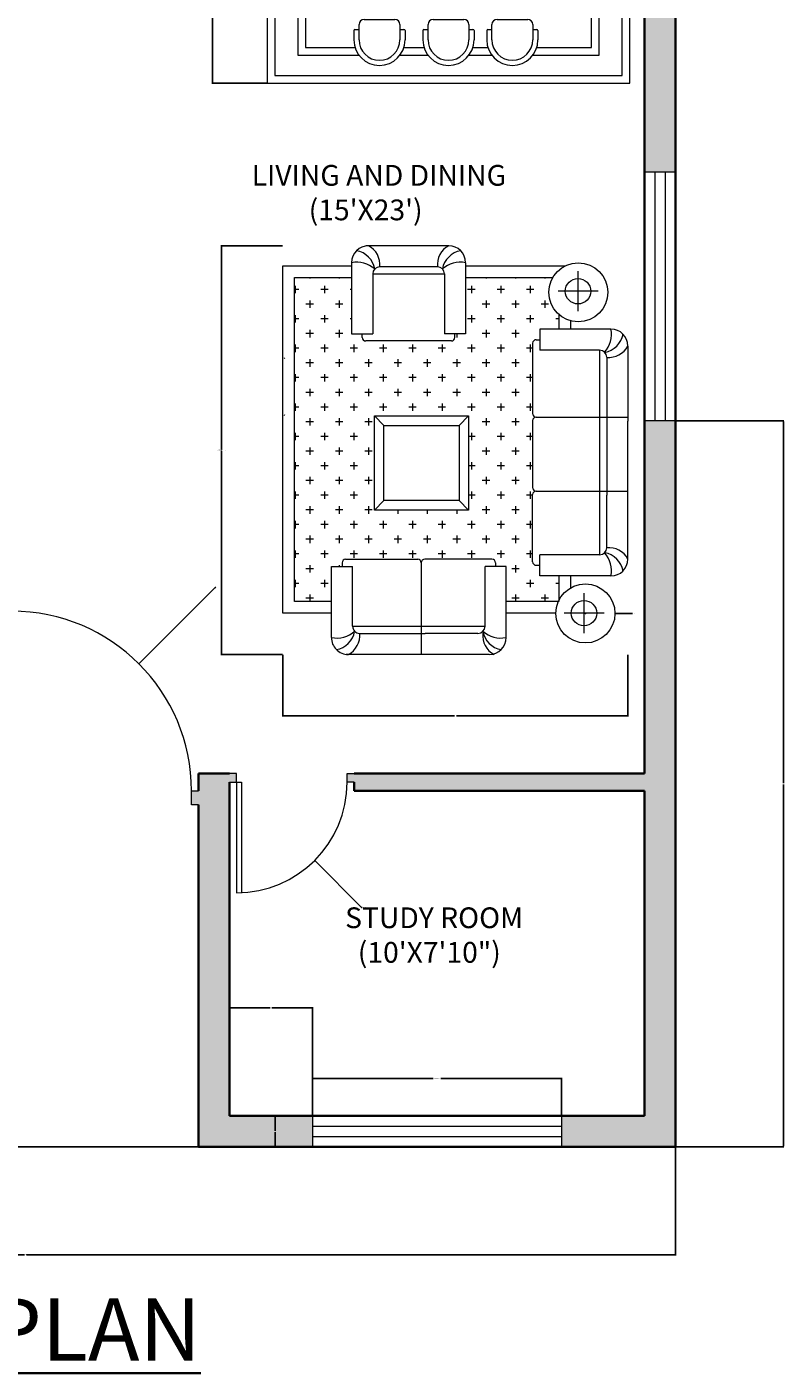
# Model space of a CAD drawing. Units: inches. Extents: x 2948 to 4025, y 2171 to 2966.
# Tile 2 of 6: x 3168 to 3387, y 2171 to 2560. Entities that reach past the tile are written whole.
import ezdxf

# ---------------------------------------------------------------- set-up
doc = ezdxf.new("R2010")
doc.units = ezdxf.units.IN
for name, color, linetype, lineweight in [('A-ANNO-DIMS', 2, 'Continuous', 18), ('A-ANNO-TEXT', 7, 'Continuous', 35), ('A-AREA-IDEN', 7, 'Continuous', 18), ('A-DOOR', 3, 'Continuous', 18), ('A-FURN', 8, 'Continuous', 18), ('A-GLAZ', 4, 'Continuous', 18), ('A-WALL', 7, 'Continuous', 35), ('A-WALL-PATT', 252, 'Continuous', 13)]:
    doc.layers.add(name, color=color, linetype=linetype, lineweight=lineweight)
doc.styles.get("Standard").update_dxf_attribs({"font": 'arial.ttf'})
doc.dimstyles.get("Standard").update_dxf_attribs({"dimtxt": 0.18, "dimasz": 0.18, "dimexe": 0.18, "dimexo": 0.0625, "dimgap": 0.09, "dimtad": 0, "dimtih": 1, "dimtoh": 1, "dimdec": 4, "dimzin": 0, "dimdsep": 46, "dimtxsty": 'Standard', "dimcen": 0.09, "dimadec": 0, "dimazin": 0, "dimtfac": 1, "dimtdec": 4, "dimtofl": 0, "dimtmove": 0, "dimatfit": 3, "dimfxl": 1, "dimtolj": 1, "dimtzin": 0, "dimarcsym": 0})

# ---------------------------------------------------------------- blocks, each defined once
blk = doc.blocks.new('A$C27801A2F')
for p, q in [((3.55, 2.425), (0, 2.425)), ((0, 2.425), (0, 0)), ((3.55, 0), (3.55, 2.425)), ((3.475, 2.35), (0.075, 2.35)), ((0.075, 2.35), (0.075, 0.075)), ((3.475, 0.075), (3.475, 2.35)), ((0.9, 2.125), (0.3, 2.125)), ((0.3, 2.125), (0.3, 1.325)), ((1.575, 2.125), (1.3, 2.125)), ((2.2, 2.125), (1.975, 2.125)), ((3.25, 2.125), (2.6, 2.125)), ((3.25, 1.325), (3.25, 2.125)), ((0.375, 2.05), (0.375, 1.392)), ((0.862, 2.05), (0.375, 2.05)), ((1.537, 2.05), (1.338, 2.05)), ((2.162, 2.05), (2.013, 2.05)), ((3.175, 2.05), (2.638, 2.05)), ((3.175, 1.392), (3.175, 2.05)), ((0.85, 1.885), (0.85, 1.975)), ((0.86, 1.875), (0.9, 1.875)), ((0.9, 1.975), (0.9, 1.825)), ((1.3, 1.825), (1.3, 1.975)), ((1.3, 1.875), (1.34, 1.875)), ((1.35, 1.885), (1.35, 1.975)), ((1.525, 1.885), (1.525, 1.975)), ((1.535, 1.875), (1.575, 1.875)), ((1.575, 1.975), (1.575, 1.825)), ((1.975, 1.825), (1.975, 1.975)), ((1.975, 1.875), (2.015, 1.875)), ((2.025, 1.885), (2.025, 1.975)), ((2.15, 1.885), (2.15, 1.975)), ((2.16, 1.875), (2.2, 1.875)), ((2.2, 1.975), (2.2, 1.825)), ((2.6, 1.825), (2.6, 1.975)), ((2.6, 1.875), (2.64, 1.875)), ((2.65, 1.885), (2.65, 1.975)), ((0.95, 1.775), (1.25, 1.775)), ((1.625, 1.775), (1.925, 1.775)), ((2.25, 1.775), (2.55, 1.775)), ((0.775, 0.7), (0.775, 1.7)), ((0.775, 1.7), (2.775, 1.7)), ((2.775, 1.7), (2.775, 0.7)), ((0.59, 1.425), (0.5, 1.425)), ((0.65, 1.375), (0.5, 1.375)), ((0.6, 1.375), (0.6, 1.415)), ((0.7, 1.025), (0.7, 1.325)), ((2.85, 1.325), (2.85, 1.025)), ((3.05, 1.375), (2.9, 1.375)), ((2.95, 1.415), (2.95, 1.375)), ((2.96, 1.425), (3.05, 1.425)), ((0.3, 1.025), (0.3, 0.275)), ((0.375, 0.958), (0.375, 0.35)), ((0.5, 0.975), (0.65, 0.975)), ((0.59, 0.925), (0.5, 0.925)), ((0.6, 0.935), (0.6, 0.975)), ((2.9, 0.975), (3.05, 0.975)), ((2.95, 0.975), (2.95, 0.935)), ((2.96, 0.925), (3.05, 0.925)), ((3.175, 0.35), (3.175, 0.958)), ((3.25, 0.275), (3.25, 1.025)), ((2.775, 0.7), (0.775, 0.7)), ((0.9, 0.425), (0.9, 0.575)), ((0.95, 0.625), (1.25, 0.625)), ((1.3, 0.575), (1.3, 0.425)), ((1.575, 0.425), (1.575, 0.575)), ((1.625, 0.625), (1.925, 0.625)), ((1.975, 0.575), (1.975, 0.425)), ((2.2, 0.425), (2.2, 0.575)), ((2.25, 0.625), (2.55, 0.625)), ((2.6, 0.575), (2.6, 0.425)), ((0.85, 0.515), (0.85, 0.425)), ((0.86, 0.525), (0.9, 0.525)), ((1.3, 0.525), (1.34, 0.525)), ((1.35, 0.515), (1.35, 0.425)), ((1.525, 0.515), (1.525, 0.425)), ((1.535, 0.525), (1.575, 0.525)), ((1.975, 0.525), (2.015, 0.525)), ((2.025, 0.515), (2.025, 0.425)), ((2.15, 0.515), (2.15, 0.425)), ((2.16, 0.525), (2.2, 0.525)), ((2.6, 0.525), (2.64, 0.525)), ((2.65, 0.515), (2.65, 0.425)), ((0.3, 0.275), (0.9, 0.275)), ((0.375, 0.35), (0.862, 0.35)), ((1.3, 0.275), (1.575, 0.275)), ((1.338, 0.35), (1.537, 0.35)), ((1.975, 0.275), (2.2, 0.275)), ((2.013, 0.35), (2.162, 0.35)), ((2.6, 0.275), (3.25, 0.275)), ((2.638, 0.35), (3.175, 0.35)), ((0, 0), (3.55, 0)), ((0.075, 0.075), (3.475, 0.075))]:
    blk.add_line(p, q)
for centre, radius, start, end in [((1.1, 1.975), 0.25, 0, 180), ((1.1, 1.975), 0.2, 0.0001, 179.9999), ((1.775, 1.975), 0.25, 0, 180), ((1.775, 1.975), 0.2, 0.0001, 179.9999), ((2.4, 1.975), 0.25, 0, 180), ((2.4, 1.975), 0.2, 0.0001, 179.9999), ((0.86, 1.885), 0.01, 180, 270), ((1.34, 1.885), 0.01, 270, 0), ((1.535, 1.885), 0.01, 180, 270), ((2.015, 1.885), 0.01, 270, 0), ((2.16, 1.885), 0.01, 180, 270), ((2.64, 1.885), 0.01, 270, 0), ((0.95, 1.825), 0.05, 180, 270), ((1.25, 1.825), 0.05, 270, 0), ((1.625, 1.825), 0.05, 180, 270), ((1.925, 1.825), 0.05, 270, 0), ((2.25, 1.825), 0.05, 180, 270), ((2.55, 1.825), 0.05, 270, 0), ((0.5, 1.175), 0.25, 90, 270), ((0.5, 1.175), 0.2, 90.0001, 269.9999), ((0.65, 1.325), 0.05, 0, 90), ((2.9, 1.325), 0.05, 90, 180), ((2.96, 1.415), 0.01, 90, 180), ((3.05, 1.175), 0.25, 270, 90), ((3.05, 1.175), 0.2, 270.0001, 89.9999), ((0.65, 1.025), 0.05, 270, 0), ((2.9, 1.025), 0.05, 180, 270), ((2.96, 0.935), 0.01, 180, 270), ((0.95, 0.575), 0.05, 90, 180), ((1.25, 0.575), 0.05, 0, 90), ((1.625, 0.575), 0.05, 90, 180), ((1.925, 0.575), 0.05, 0, 90), ((2.25, 0.575), 0.05, 90, 180), ((2.55, 0.575), 0.05, 0, 90), ((0.86, 0.515), 0.01, 90, 180), ((1.1, 0.425), 0.25, 180, 0), ((1.1, 0.425), 0.2, 180.0001, 359.9999), ((1.34, 0.515), 0.01, 0, 90), ((1.535, 0.515), 0.01, 90, 180), ((1.775, 0.425), 0.25, 180, 0), ((1.775, 0.425), 0.2, 180.0001, 359.9999), ((2.015, 0.515), 0.01, 0, 90), ((2.16, 0.515), 0.01, 90, 180), ((2.4, 0.425), 0.25, 180, 0), ((2.4, 0.425), 0.2, 180.0001, 359.9999), ((2.64, 0.515), 0.01, 0, 90)]:
    blk.add_arc(centre, radius, start, end)
blk = doc.blocks.new('A$C305E417A')
for p, q in [((853, 2935), (1492, 2935)), ((1458, 2155), (1458, 2935)), ((1458, 2155), (1458, 2935)), ((2665, 2935), (1492, 2935)), ((2087, 2155), (2087, 2935)), ((709, 2791), (709, 2186)), ((949, 2755), (2121, 2755)), ((2569, 2755), (2121, 2755)), ((2809, 2791), (2809, 2186)), ((387, 2681), (387, 2341)), ((889, 2695), (2629, 2695)), ((889, 2695), (889, 2186)), ((2629, 2695), (2629, 2186)), ((3125, 2732), (3125, 2392)), ((3295, 2562), (2955, 2562)), ((557, 2511), (217, 2511)), ((639, 2448), (709, 2448)), ((2809, 2448), (2910, 2448)), ((171, 1555), (171, 2401)), ((270, 1555), (270, 2295)), ((586, 2349), (709, 2349)), ((622, 2349), (622, 2322)), ((2809, 2349), (3025, 2349)), ((2872, 2349), (2872, 2322)), ((3025, 2349), (3025, 1900)), ((3125, 2322), (3125, 1900)), ((270, 2229), (279, 2229)), ((466, 2229), (529, 2229)), ((497, 2260), (497, 2197)), ((709, 2186), (889, 2186)), ((799, 2155), (799, 2186)), ((2809, 2186), (2629, 2186)), ((2718, 2155), (2718, 2186)), ((2966, 2229), (3025, 2229)), ((2997, 2260), (2997, 2197)), ((341, 2104), (404, 2104)), ((372, 2135), (372, 2072)), ((591, 2104), (654, 2104)), ((622, 2135), (622, 2072)), ((829, 2125), (1428, 2125)), ((841, 2104), (904, 2104)), ((872, 2125), (872, 2072)), ((1091, 2104), (1154, 2104)), ((1122, 2125), (1122, 2072)), ((1341, 2104), (1404, 2104)), ((1372, 2125), (1372, 2072)), ((1488, 2125), (2057, 2125)), ((1591, 2104), (1654, 2104)), ((1622, 2125), (1622, 2072)), ((1841, 2104), (1904, 2104)), ((1872, 2125), (1872, 2072)), ((2091, 2104), (2154, 2104)), ((2688, 2125), (2117, 2125)), ((2122, 2125), (2122, 2072)), ((2341, 2104), (2404, 2104)), ((2372, 2125), (2372, 2072)), ((2591, 2104), (2654, 2104)), ((2622, 2125), (2622, 2072)), ((2841, 2104), (2904, 2104)), ((2872, 2135), (2872, 2072)), ((270, 1979), (279, 1979)), ((466, 1979), (529, 1979)), ((497, 2010), (497, 1947)), ((716, 1979), (779, 1979)), ((747, 2010), (747, 1947)), ((966, 1979), (1029, 1979)), ((997, 2010), (997, 1947)), ((1216, 1979), (1279, 1979)), ((1247, 2010), (1247, 1947)), ((1466, 1979), (1529, 1979)), ((1497, 2010), (1497, 1947)), ((1716, 1979), (1779, 1979)), ((1747, 2010), (1747, 1947)), ((1966, 1979), (2029, 1979)), ((1997, 2010), (1997, 1947)), ((2216, 1979), (2279, 1979)), ((2247, 2010), (2247, 1947)), ((2466, 1979), (2529, 1979)), ((2497, 2010), (2497, 1947)), ((2716, 1979), (2779, 1979)), ((2747, 2010), (2747, 1947)), ((2966, 1979), (3025, 1979)), ((2997, 2010), (2997, 1947)), ((341, 1854), (404, 1854)), ((372, 1885), (372, 1822)), ((591, 1854), (654, 1854)), ((622, 1885), (622, 1822)), ((841, 1854), (904, 1854)), ((872, 1885), (872, 1822)), ((1091, 1854), (1154, 1854)), ((1122, 1885), (1122, 1822)), ((1341, 1854), (1404, 1854)), ((1372, 1885), (1372, 1822)), ((1591, 1854), (1654, 1854)), ((1622, 1885), (1622, 1822)), ((1841, 1854), (1904, 1854)), ((1872, 1885), (1872, 1822)), ((2091, 1854), (2154, 1854)), ((2122, 1885), (2122, 1822)), ((2341, 1854), (2404, 1854)), ((2372, 1885), (2372, 1822)), ((2591, 1854), (2654, 1854)), ((2622, 1885), (2622, 1822)), ((3333, 1900), (2728, 1900)), ((2728, 1900), (2728, 1720)), ((270, 1729), (279, 1729)), ((466, 1729), (529, 1729)), ((497, 1760), (497, 1697)), ((716, 1729), (779, 1729)), ((747, 1760), (747, 1697)), ((966, 1729), (1029, 1729)), ((997, 1760), (997, 1697)), ((1216, 1729), (1279, 1729)), ((1247, 1760), (1247, 1697)), ((1466, 1729), (1529, 1729)), ((1497, 1760), (1497, 1697)), ((1716, 1729), (1779, 1729)), ((1747, 1760), (1747, 1697)), ((1966, 1729), (2029, 1729)), ((1997, 1760), (1997, 1697)), ((2216, 1729), (2279, 1729)), ((2247, 1760), (2247, 1697)), ((2466, 1729), (2529, 1729)), ((2497, 1760), (2497, 1697)), ((2667, 1779), (2667, 1207)), ((2697, 1809), (2728, 1809)), ((3237, 1720), (2728, 1720)), ((3237, 593), (3237, 1720)), ((3477, 1756), (3477, 538)), ((341, 1604), (404, 1604)), ((372, 1635), (372, 1572)), ((591, 1604), (654, 1604)), ((622, 1635), (622, 1572)), ((841, 1604), (904, 1604)), ((872, 1635), (872, 1572)), ((1091, 1604), (1154, 1604)), ((1122, 1635), (1122, 1572)), ((1341, 1604), (1404, 1604)), ((1372, 1635), (1372, 1572)), ((1591, 1604), (1654, 1604)), ((1622, 1635), (1622, 1580)), ((1841, 1604), (1904, 1604)), ((1872, 1635), (1872, 1580)), ((2091, 1604), (2154, 1604)), ((2122, 1635), (2122, 1580)), ((2341, 1604), (2404, 1604)), ((2372, 1635), (2372, 1572)), ((2591, 1604), (2654, 1604)), ((2622, 1635), (2622, 1572)), ((3297, 1660), (3297, 1212)), ((144, 1555), (749, 1555)), ((749, 1555), (749, 1375)), ((997, 1510), (997, 1447)), ((1247, 1510), (1247, 1447)), ((1448, 780), (1448, 1580)), ((1448, 1580), (2248, 1580)), ((1528, 1500), (1448, 1580)), ((1528, 860), (1528, 1500)), ((1528, 1500), (2168, 1500)), ((2168, 1500), (2248, 1580)), ((2168, 1500), (2168, 860)), ((2248, 1580), (2248, 780)), ((2497, 1510), (2497, 1447)), ((0, 1411), (0, 710)), ((240, 765), (240, 1375)), ((240, 1375), (749, 1375)), ((749, 1479), (779, 1479)), ((780, 1464), (749, 1464)), ((810, 1434), (810, 705)), ((872, 1385), (872, 1322)), ((966, 1479), (1029, 1479)), ((1122, 1385), (1122, 1322)), ((1216, 1479), (1279, 1479)), ((1372, 1385), (1372, 1322)), ((2248, 1479), (2279, 1479)), ((2372, 1385), (2372, 1322)), ((2466, 1479), (2529, 1479)), ((2622, 1385), (2622, 1322)), ((180, 1315), (180, 825)), ((841, 1354), (904, 1354)), ((997, 1260), (997, 1197)), ((1091, 1354), (1154, 1354)), ((1247, 1260), (1247, 1197)), ((1341, 1354), (1404, 1354)), ((2341, 1354), (2404, 1354)), ((2497, 1260), (2497, 1197)), ((2591, 1354), (2654, 1354)), ((966, 1229), (1029, 1229)), ((1216, 1229), (1279, 1229)), ((2248, 1229), (2279, 1229)), ((2466, 1229), (2529, 1229)), ((2667, 534), (2667, 1147)), ((2697, 1177), (3477, 1177)), ((3297, 653), (3297, 1212)), ((841, 1104), (904, 1104)), ((872, 1135), (872, 1072)), ((1091, 1104), (1154, 1104)), ((1122, 1135), (1122, 1072)), ((1341, 1104), (1404, 1104)), ((1372, 1135), (1372, 1072)), ((2341, 1104), (2404, 1104)), ((2372, 1135), (2372, 1072)), ((2591, 1104), (2654, 1104)), ((2622, 1135), (2622, 1072)), ((966, 979), (1029, 979)), ((997, 1010), (997, 947)), ((1216, 979), (1279, 979)), ((1247, 1010), (1247, 947)), ((2248, 979), (2279, 979)), ((2466, 979), (2529, 979)), ((2497, 1010), (2497, 947)), ((841, 854), (904, 854)), ((872, 885), (872, 822)), ((1091, 854), (1154, 854)), ((1122, 885), (1122, 822)), ((1341, 854), (1404, 854)), ((1372, 885), (1372, 822)), ((1528, 860), (1448, 780)), ((2168, 860), (1528, 860)), ((2168, 860), (2248, 780)), ((2341, 854), (2404, 854)), ((2372, 885), (2372, 822)), ((2591, 854), (2654, 854)), ((2622, 885), (2622, 822)), ((0, 729), (0, 710)), ((240, 765), (749, 765)), ((749, 585), (749, 765)), ((966, 729), (1029, 729)), ((997, 760), (997, 697)), ((1216, 729), (1279, 729)), ((1247, 760), (1247, 697)), ((2248, 780), (1448, 780)), ((1466, 729), (1529, 729)), ((1497, 760), (1497, 697)), ((1716, 729), (1779, 729)), ((1747, 760), (1747, 697)), ((1966, 729), (2029, 729)), ((1997, 760), (1997, 697)), ((2216, 729), (2279, 729)), ((2247, 760), (2247, 697)), ((2466, 729), (2529, 729)), ((2497, 760), (2497, 697)), ((144, 585), (749, 585)), ((171, 0), (171, 585)), ((270, 100), (270, 585)), ((372, 585), (372, 572)), ((622, 585), (622, 572)), ((780, 675), (749, 675)), ((841, 604), (904, 604)), ((872, 635), (872, 572)), ((1091, 604), (1154, 604)), ((1122, 635), (1122, 572)), ((1341, 604), (1404, 604)), ((1372, 635), (1372, 572)), ((1591, 604), (1654, 604)), ((1622, 635), (1622, 572)), ((1841, 604), (1904, 604)), ((1872, 635), (1872, 572)), ((2091, 604), (2154, 604)), ((2122, 635), (2122, 572)), ((2341, 604), (2404, 604)), ((2372, 635), (2372, 572)), ((2591, 604), (2654, 604)), ((2622, 635), (2622, 572)), ((3237, 593), (2728, 593)), ((2728, 413), (2728, 593)), ((270, 479), (279, 479)), ((466, 479), (529, 479)), ((497, 510), (497, 447)), ((716, 479), (779, 479)), ((747, 510), (747, 447)), ((966, 479), (1029, 479)), ((997, 510), (997, 447)), ((1216, 479), (1279, 479)), ((1247, 510), (1247, 447)), ((1466, 479), (1529, 479)), ((1497, 510), (1497, 447)), ((1716, 479), (1779, 479)), ((1747, 510), (1747, 447)), ((1966, 479), (2029, 479)), ((1997, 510), (1997, 447)), ((2216, 479), (2279, 479)), ((2247, 510), (2247, 447)), ((2466, 479), (2529, 479)), ((2497, 510), (2497, 447)), ((2697, 504), (2728, 504)), ((2716, 479), (2728, 479)), ((3477, 557), (3477, 538)), ((341, 354), (404, 354)), ((372, 385), (372, 322)), ((591, 354), (654, 354)), ((622, 385), (622, 322)), ((841, 354), (904, 354)), ((872, 385), (872, 322)), ((1091, 354), (1154, 354)), ((1122, 385), (1122, 322)), ((1341, 354), (1404, 354)), ((1372, 385), (1372, 322)), ((1591, 354), (1654, 354)), ((1622, 385), (1622, 322)), ((1841, 354), (1904, 354)), ((1872, 385), (1872, 322)), ((2091, 354), (2154, 354)), ((2122, 385), (2122, 322)), ((2341, 354), (2404, 354)), ((2372, 385), (2372, 322)), ((2591, 354), (2654, 354)), ((2622, 385), (2622, 322)), ((3333, 413), (2728, 413)), ((2841, 354), (2904, 354)), ((2872, 385), (2872, 322)), ((3025, 413), (3025, 100)), ((3125, 413), (3125, 0)), ((497, 260), (497, 197)), ((747, 260), (747, 197)), ((997, 260), (997, 197)), ((1247, 260), (1247, 197)), ((1497, 260), (1497, 197)), ((1747, 260), (1747, 197)), ((1997, 260), (1997, 197)), ((2247, 260), (2247, 197)), ((2497, 260), (2497, 197)), ((2747, 260), (2747, 197)), ((2997, 260), (2997, 197)), ((270, 229), (279, 229)), ((372, 135), (372, 100)), ((466, 229), (529, 229)), ((622, 135), (622, 100)), ((716, 229), (779, 229)), ((872, 135), (872, 100)), ((966, 229), (1029, 229)), ((1122, 135), (1122, 100)), ((1216, 229), (1279, 229)), ((1372, 135), (1372, 100)), ((1466, 229), (1529, 229)), ((1622, 135), (1622, 100)), ((1716, 229), (1779, 229)), ((1872, 135), (1872, 100)), ((1966, 229), (2029, 229)), ((2122, 135), (2122, 100)), ((2216, 229), (2279, 229)), ((2372, 135), (2372, 100)), ((2466, 229), (2529, 229)), ((2622, 135), (2622, 100)), ((2716, 229), (2779, 229)), ((2872, 135), (2872, 100)), ((2966, 229), (3025, 229)), ((3125, 0), (171, 0)), ((3025, 100), (270, 100)), ((341, 104), (404, 104)), ((591, 104), (654, 104)), ((841, 104), (904, 104)), ((1091, 104), (1154, 104)), ((1341, 104), (1404, 104)), ((1591, 104), (1654, 104)), ((1841, 104), (1904, 104)), ((2091, 104), (2154, 104)), ((2341, 104), (2404, 104)), ((2591, 104), (2654, 104)), ((2841, 104), (2904, 104))]:
    blk.add_line(p, q)
for centre, radius in [((396, 2513), 251), ((3128, 2574), 251), ((3125, 2562), 108), ((387, 2511), 108)]:
    blk.add_circle(centre, radius)
for centre, radius, start, end in [((853, 2791), 144, 90, 180), ((716, 2703), 194, 10.4091, 79.5909), ((764, 2772), 186, 354.7206, 61.4244), ((2754, 2772), 186, 118.5756, 185.2794), ((2802, 2703), 194, 100.4091, 169.5909), ((2665, 2791), 144, 0, 90), ((752, 2560), 235, 49.0321, 100.6252), ((949, 2695), 60, 90, 180), ((2569, 2695), 60, 0, 90), ((2766, 2560), 235, 79.3748, 130.9679), ((829, 2155), 30, 180, 270), ((1428, 2155), 30, 270, 0), ((1488, 2155), 30, 180, 270), ((2057, 2155), 30, 270, 0), ((2117, 2155), 30, 180, 270), ((2688, 2155), 30, 270, 0), ((3102, 1856), 235, 319.0321, 10.6252), ((3245, 1892), 194, 280.4091, 349.5909), ((3333, 1756), 144, 0, 90), ((2697, 1779), 30, 90, 180), ((3237, 1660), 60, 0, 90), ((3314, 1886), 186, 264.7206, 331.4244), ((144, 1411), 144, 90, 180), ((233, 1548), 194, 190.4091, 259.5909), ((375, 1511), 235, 169.3748, 220.9679), ((163, 1500), 186, 208.5756, 275.2794), ((240, 1315), 60, 90, 180), ((780, 1434), 30, 0, 90), ((2697, 1207), 30, 180, 270), ((2697, 1147), 30, 90, 180), ((163, 640), 186, 84.7206, 151.4244), ((240, 825), 60, 180, 270), ((144, 729), 144, 180, 270), ((233, 592), 194, 100.4091, 169.5909), ((375, 628), 235, 139.0321, 190.6252), ((780, 705), 30, 270, 0), ((3237, 653), 60, 270, 0), ((3102, 457), 235, 349.3748, 40.9679), ((3245, 420), 194, 10.4091, 79.5909), ((3314, 469), 186, 28.5756, 95.2794), ((2697, 534), 30, 180, 270), ((3333, 557), 144, 270, 0), ((961, 6), 10, 90, 135), ((1436, 6), 10, 45, 90)]:
    blk.add_arc(centre, radius, start, end)
blk = doc.blocks.new('DOOR-SWING-32IN')
for p, q in [((2, 34.5), (0, 34.5)), ((0, 32), (2, 32)), ((2, 32), (2, 34.5)), ((2, 32), (2, 0)), ((2, 32), (3.5, 32)), ((3.5, 32), (3.5, 0.04)), ((34, 32), (34, 34.5)), ((34, 34.5), (36, 34.5)), ((36, 32), (34, 32))]:
    blk.add_line(p, q)
blk.add_arc((2, 32), 32, 270, 0)
blk = doc.blocks.new('DOOR-ENTRY-52IN')
for p, q in [((2, 4), (2, 56)), ((3.5, 4), (3.5, 55.98)), ((2, 4), (0, 4)), ((2, 0), (2, 4)), ((2, 4), (3.5, 4)), ((54, 0), (54, 4)), ((54, 4), (56, 4)), ((0, 0), (2, 0)), ((56, 0), (54, 0))]:
    blk.add_line(p, q)
blk.add_arc((2, 4), 52, 0, 90)
blk = doc.blocks.new('WIN-72IN')
for p, q in [((0, 0), (0, 9)), ((72, 0), (72, 9)), ((72, 6), (0, 6)), ((72, 3), (0, 3))]:
    blk.add_line(p, q)
blk = doc.blocks.new('*D21')
at = {"layer": 'A-ANNO-DIMS', "color": 0, "lineweight": -2, "transparency": 16777216}
for p, q in [((3250.51, 2245.05), (3250.51, 2255.97)), ((3250.69, 2255.79), (3285.4, 2255.79)), ((3322.33, 2255.79), (3287.63, 2255.79)), ((3322.51, 2245.05), (3322.51, 2255.97))]:
    blk.add_line(p, q, dxfattribs=at)
at = {"layer": 'A-ANNO-DIMS', "color": 0, "transparency": 16777216}
for points in [[(3250.69, 2255.82), (3250.69, 2255.76), (3250.51, 2255.79)], [(3322.33, 2255.82), (3322.33, 2255.76), (3322.51, 2255.79)]]:
    blk.add_solid(points, dxfattribs=at)
at = {"layer": 'Defpoints', "color": 0, "transparency": 16777216}
for p in [(3250.51, 2255.79), (3250.51, 2244.99), (3322.51, 2244.99)]:
    blk.add_point(p, dxfattribs=at)
at = {"layer": 'A-ANNO-DIMS', "color": 0, "transparency": 16777216, "insert": (3286.51, 2255.79), "char_height": 0.18, "attachment_point": 5}
blk.add_mtext('\\A1;WINDOW 72 TYP.', dxfattribs=at)
blk = doc.blocks.new('*D22')
at = {"layer": 'A-ANNO-DIMS', "color": 0, "lineweight": -2, "transparency": 16777216}
for p, q in [((3250.45, 2244.99), (3239.53, 2244.99)), ((3239.71, 2244.81), (3239.71, 2240.67)), ((3239.71, 2236.17), (3239.71, 2240.3)), ((3250.45, 2235.99), (3239.53, 2235.99))]:
    blk.add_line(p, q, dxfattribs=at)
at = {"layer": 'A-ANNO-DIMS', "color": 0, "transparency": 16777216}
for points in [[(3239.68, 2244.81), (3239.74, 2244.81), (3239.71, 2244.99)], [(3239.68, 2236.17), (3239.74, 2236.17), (3239.71, 2235.99)]]:
    blk.add_solid(points, dxfattribs=at)
at = {"layer": 'Defpoints', "color": 0, "transparency": 16777216}
for p in [(3250.51, 2244.99), (3239.71, 2235.99), (3250.51, 2235.99)]:
    blk.add_point(p, dxfattribs=at)
at = {"layer": 'A-ANNO-DIMS', "color": 0, "transparency": 16777216, "insert": (3239.71, 2240.49), "char_height": 0.18, "attachment_point": 5}
blk.add_mtext('\\A1;9 TYP.', dxfattribs=at)
blk = doc.blocks.new('*D30')
at = {"layer": 'A-ANNO-DIMS', "color": 0, "lineweight": -2, "transparency": 16777216}
for p, q in [((3237.3, 2615.38), (3221.43, 2615.38)), ((3221.61, 2615.2), (3221.61, 2579.71)), ((3221.61, 2543.86), (3221.61, 2579.35)), ((3237.3, 2543.68), (3221.43, 2543.68))]:
    blk.add_line(p, q, dxfattribs=at)
at = {"layer": 'A-ANNO-DIMS', "color": 0, "transparency": 16777216}
for points in [[(3221.58, 2615.2), (3221.64, 2615.2), (3221.61, 2615.38)], [(3221.58, 2543.86), (3221.64, 2543.86), (3221.61, 2543.68)]]:
    blk.add_solid(points, dxfattribs=at)
at = {"layer": 'Defpoints', "color": 0, "transparency": 16777216}
for p in [(3221.61, 2615.38), (3237.36, 2615.38), (3237.36, 2543.68)]:
    blk.add_point(p, dxfattribs=at)
at = {"layer": 'A-ANNO-DIMS', "color": 0, "transparency": 16777216, "insert": (3221.61, 2579.53), "char_height": 0.18, "attachment_point": 5}
blk.add_mtext('\\A1;72', dxfattribs=at)
blk = doc.blocks.new('*D31')
at = {"layer": 'A-ANNO-DIMS', "color": 0, "lineweight": -2, "transparency": 16777216}
for p, q in [((3241.86, 2496.68), (3224.01, 2496.68)), ((3224.19, 2496.5), (3224.19, 2437.74)), ((3224.19, 2378.61), (3224.19, 2437.37)), ((3241.86, 2378.43), (3224.01, 2378.43))]:
    blk.add_line(p, q, dxfattribs=at)
at = {"layer": 'A-ANNO-DIMS', "color": 0, "transparency": 16777216}
for points in [[(3224.16, 2496.5), (3224.22, 2496.5), (3224.19, 2496.68)], [(3224.16, 2378.61), (3224.22, 2378.61), (3224.19, 2378.43)]]:
    blk.add_solid(points, dxfattribs=at)
at = {"layer": 'Defpoints', "color": 0, "transparency": 16777216}
for p in [(3241.92, 2496.68), (3224.19, 2378.43), (3241.92, 2378.43)]:
    blk.add_point(p, dxfattribs=at)
at = {"layer": 'A-ANNO-DIMS', "color": 0, "transparency": 16777216, "insert": (3224.19, 2437.56), "char_height": 0.18, "attachment_point": 5}
blk.add_mtext('\\A1;SEATING GROUP 118', dxfattribs=at)
blk = doc.blocks.new('*D32')
at = {"layer": 'A-ANNO-DIMS', "color": 0, "lineweight": -2, "transparency": 16777216}
for p, q in [((3241.92, 2378.37), (3241.92, 2360.52)), ((3341.75, 2378.37), (3341.75, 2360.52)), ((3242.1, 2360.7), (3291.56, 2360.7)), ((3341.57, 2360.7), (3292.12, 2360.7))]:
    blk.add_line(p, q, dxfattribs=at)
at = {"layer": 'A-ANNO-DIMS', "color": 0, "transparency": 16777216}
for points in [[(3242.1, 2360.73), (3242.1, 2360.67), (3241.92, 2360.7)], [(3341.57, 2360.73), (3341.57, 2360.67), (3341.75, 2360.7)]]:
    blk.add_solid(points, dxfattribs=at)
at = {"layer": 'Defpoints', "color": 0, "transparency": 16777216}
for p in [(3241.92, 2378.43), (3341.75, 2378.43), (3341.75, 2360.7)]:
    blk.add_point(p, dxfattribs=at)
at = {"layer": 'A-ANNO-DIMS', "color": 0, "transparency": 16777216, "insert": (3291.84, 2360.7), "char_height": 0.18, "attachment_point": 5}
blk.add_mtext('\\A1;100', dxfattribs=at)
blk = doc.blocks.new('*D37')
at = {"layer": 'A-ANNO-DIMS', "color": 0, "lineweight": -2, "transparency": 16777216}
for p, q in [((2979.51, 2334.92), (2979.51, 2204.61)), ((3355.51, 2235.92), (3355.51, 2204.61)), ((2979.69, 2204.79), (3167.22, 2204.79)), ((3355.33, 2204.79), (3167.8, 2204.79))]:
    blk.add_line(p, q, dxfattribs=at)
at = {"layer": 'A-ANNO-DIMS', "color": 0, "transparency": 16777216}
for points in [[(2979.69, 2204.82), (2979.69, 2204.76), (2979.51, 2204.79)], [(3355.33, 2204.82), (3355.33, 2204.76), (3355.51, 2204.79)]]:
    blk.add_solid(points, dxfattribs=at)
at = {"layer": 'Defpoints', "color": 0, "transparency": 16777216}
for p in [(2979.51, 2334.99), (3355.51, 2235.99), (3355.51, 2204.79)]:
    blk.add_point(p, dxfattribs=at)
at = {"layer": 'A-ANNO-DIMS', "color": 0, "transparency": 16777216, "insert": (3167.51, 2204.79), "char_height": 0.18, "attachment_point": 5}
blk.add_mtext('\\A1;376', dxfattribs=at)
blk = doc.blocks.new('*D38')
at = {"layer": 'A-ANNO-DIMS', "color": 0, "lineweight": -2, "transparency": 16777216}
for p, q in [((2979.45, 2777.99), (2948.13, 2777.99)), ((2948.31, 2777.81), (2948.31, 2507.17)), ((2948.31, 2236.17), (2948.31, 2506.8)), ((3217.45, 2235.99), (2948.13, 2235.99))]:
    blk.add_line(p, q, dxfattribs=at)
at = {"layer": 'A-ANNO-DIMS', "color": 0, "transparency": 16777216}
for points in [[(2948.28, 2777.81), (2948.34, 2777.81), (2948.31, 2777.99)], [(2948.28, 2236.17), (2948.34, 2236.17), (2948.31, 2235.99)]]:
    blk.add_solid(points, dxfattribs=at)
at = {"layer": 'Defpoints', "color": 0, "transparency": 16777216}
for p in [(2948.31, 2777.99), (2979.51, 2777.99), (3217.51, 2235.99)]:
    blk.add_point(p, dxfattribs=at)
at = {"layer": 'A-ANNO-DIMS', "color": 0, "transparency": 16777216, "insert": (2948.31, 2506.99), "char_height": 0.18, "attachment_point": 5}
blk.add_mtext('\\A1;542', dxfattribs=at)
blk = doc.blocks.new('*D44')
at = {"layer": 'A-ANNO-DIMS', "color": 0, "lineweight": -2, "transparency": 16777216}
for p, q in [((3355.58, 2445.99), (3386.89, 2445.99)), ((3386.71, 2445.81), (3386.71, 2341.17)), ((3386.71, 2236.17), (3386.71, 2340.8)), ((3355.58, 2235.99), (3386.89, 2235.99))]:
    blk.add_line(p, q, dxfattribs=at)
at = {"layer": 'A-ANNO-DIMS', "color": 0, "transparency": 16777216}
for points in [[(3386.68, 2445.81), (3386.74, 2445.81), (3386.71, 2445.99)], [(3386.68, 2236.17), (3386.74, 2236.17), (3386.71, 2235.99)]]:
    blk.add_solid(points, dxfattribs=at)
at = {"layer": 'Defpoints', "color": 0, "transparency": 16777216}
for p in [(3355.51, 2445.99), (3386.71, 2445.99), (3355.51, 2235.99)]:
    blk.add_point(p, dxfattribs=at)
at = {"layer": 'A-ANNO-DIMS', "color": 0, "transparency": 16777216, "insert": (3386.71, 2340.99), "char_height": 0.18, "attachment_point": 5}
blk.add_mtext('\\A1;210', dxfattribs=at)
blk = doc.blocks.new('*D45')
at = {"layer": 'A-ANNO-DIMS', "color": 0, "lineweight": -2, "transparency": 16777216}
for p, q in [((3226.51, 2245.05), (3226.51, 2276.37)), ((3226.69, 2276.19), (3238.29, 2276.19)), ((3250.33, 2276.19), (3238.73, 2276.19)), ((3250.51, 2245.05), (3250.51, 2276.37))]:
    blk.add_line(p, q, dxfattribs=at)
at = {"layer": 'A-ANNO-DIMS', "color": 0, "transparency": 16777216}
for points in [[(3226.69, 2276.22), (3226.69, 2276.16), (3226.51, 2276.19)], [(3250.33, 2276.22), (3250.33, 2276.16), (3250.51, 2276.19)]]:
    blk.add_solid(points, dxfattribs=at)
at = {"layer": 'Defpoints', "color": 0, "transparency": 16777216}
for p in [(3250.51, 2276.19), (3226.51, 2244.99), (3250.51, 2244.99)]:
    blk.add_point(p, dxfattribs=at)
at = {"layer": 'A-ANNO-DIMS', "color": 0, "transparency": 16777216, "insert": (3238.51, 2276.19), "char_height": 0.18, "attachment_point": 5}
blk.add_mtext('\\A1;24', dxfattribs=at)
blk = doc.blocks.new('*D67')
at = {"layer": 'A-ANNO-DIMS', "color": 0, "lineweight": -2, "transparency": 16777216}
for p, q in [((3222.34, 2397.82), (3200.41, 2375.88)), ((3222.52, 2397.82), (3222.34, 2397.82)), ((3163.42, 2338.99), (3163.6, 2338.99)), ((3163.51, 2338.9), (3163.51, 2339.08))]:
    blk.add_line(p, q, dxfattribs=at)
at = {"layer": 'A-ANNO-DIMS', "color": 0, "transparency": 16777216}
blk.add_solid([(3200.39, 2375.9), (3200.43, 2375.86), (3200.28, 2375.76)], dxfattribs=at)
at = {"layer": 'Defpoints', "color": 0, "transparency": 16777216}
for p in [(3200.28, 2375.76), (3163.51, 2338.99)]:
    blk.add_point(p, dxfattribs=at)
at = {"layer": 'A-ANNO-DIMS', "color": 0, "transparency": 16777216, "insert": (3222.83, 2397.82), "char_height": 0.18, "attachment_point": 5}
blk.add_mtext('\\A1;R52', dxfattribs=at)
blk = doc.blocks.new('*D68')
at = {"layer": 'A-ANNO-DIMS', "color": 0, "lineweight": -2, "transparency": 16777216}
for p, q in [((3228.42, 2341.49), (3228.6, 2341.49)), ((3228.51, 2341.4), (3228.51, 2341.58)), ((3264.72, 2305.28), (3251.27, 2318.73)), ((3264.9, 2305.28), (3264.72, 2305.28))]:
    blk.add_line(p, q, dxfattribs=at)
at = {"layer": 'A-ANNO-DIMS', "color": 0, "transparency": 16777216}
blk.add_solid([(3251.29, 2318.75), (3251.25, 2318.71), (3251.14, 2318.86)], dxfattribs=at)
at = {"layer": 'Defpoints', "color": 0, "transparency": 16777216}
for p in [(3228.51, 2341.49), (3251.14, 2318.86)]:
    blk.add_point(p, dxfattribs=at)
at = {"layer": 'A-ANNO-DIMS', "color": 0, "transparency": 16777216, "insert": (3265.4, 2305.28), "char_height": 0.18, "attachment_point": 5}
blk.add_mtext('\\A1;4X R32', dxfattribs=at)
blk = doc.blocks.new('*D70')
at = {"layer": 'A-ANNO-DIMS', "color": 0, "lineweight": -2, "transparency": 16777216}
for p, q in [((3329.35, 2390.3), (3329.53, 2390.3)), ((3329.44, 2390.21), (3329.44, 2390.39)), ((3343.12, 2390.3), (3338.17, 2390.3))]:
    blk.add_line(p, q, dxfattribs=at)
at = {"layer": 'A-ANNO-DIMS', "color": 0, "transparency": 16777216}
blk.add_solid([(3338.17, 2390.33), (3338.17, 2390.27), (3337.99, 2390.3)], dxfattribs=at)
at = {"layer": 'Defpoints', "color": 0, "transparency": 16777216}
for p in [(3320.89, 2390.3), (3337.99, 2390.3)]:
    blk.add_point(p, dxfattribs=at)
at = {"layer": 'A-ANNO-DIMS', "color": 0, "transparency": 16777216, "insert": (3343.88, 2390.3), "char_height": 0.18, "attachment_point": 5}
blk.add_mtext('\\A1;2X ∅17.102', dxfattribs=at)

msp = doc.modelspace()

# ---------------------------------------------------------------- hatches: boundary and pattern name
at = {"layer": 'A-WALL-PATT'}
h = msp.add_hatch(color=256, dxfattribs=at)
h.dxf.hatch_style = 1
h.paths.add_polyline_path([(3355.5136, 2777.9862), (3321.0136, 2777.9862), (3321.0136, 2768.9862), (3346.5136, 2768.9862), (3346.5136, 2624.9862), (3221.0136, 2624.9862), (3221.0136, 2626.9862), (3218.5136, 2626.9862), (3218.5136, 2624.9862), (3218.5136, 2619.9862), (3346.5136, 2619.9862), (3346.5136, 2517.9862), (3355.5136, 2517.9862)])
h = msp.add_hatch(color=256, dxfattribs=at)
h.dxf.hatch_style = 1
h.paths.add_polyline_path([(3355.5136, 2445.9862), (3346.5136, 2445.9862), (3346.5136, 2343.9862), (3262.5136, 2343.9862), (3260.5136, 2343.9862), (3260.5136, 2341.4862), (3262.5136, 2341.4862), (3262.5136, 2338.9862), (3346.5136, 2338.9862), (3346.5136, 2244.9862), (3322.5136, 2244.9862), (3322.5136, 2235.9862), (3355.5136, 2235.9862)])
h = msp.add_hatch(color=256, dxfattribs=at)
h.dxf.hatch_style = 1
h.paths.add_polyline_path([(3226.5136, 2341.4862), (3228.5136, 2341.4862), (3228.5136, 2343.9862), (3226.5136, 2343.9862), (3217.5136, 2343.9862), (3217.5136, 2338.9862), (3215.5136, 2338.9862), (3215.5136, 2334.9862), (3217.5136, 2334.9862), (3217.5136, 2235.9862), (3250.5136, 2235.9862), (3250.5136, 2244.9862), (3226.5136, 2244.9862)])

# ---------------------------------------------------------------- linework, layer by layer
at = {"layer": 'A-WALL'}
for p, q in [((3355.5136, 2777.9862), (3355.5136, 2235.9862)), ((3346.5136, 2619.9862), (3346.5136, 2343.9862)), ((3217.5136, 2343.9862), (3217.5136, 2338.9862)), ((3217.5136, 2343.9862), (3226.5136, 2343.9862)), ((3226.5136, 2341.4862), (3226.5136, 2244.9862)), ((3262.5136, 2343.9862), (3346.5136, 2343.9862)), ((3262.5136, 2341.4862), (3262.5136, 2338.9862)), ((3262.5136, 2338.9862), (3346.5136, 2338.9862)), ((3346.5136, 2338.9862), (3346.5136, 2244.9862)), ((3217.5136, 2334.9862), (3217.5136, 2235.9862)), ((3226.5136, 2244.9862), (3346.5136, 2244.9862)), ((3217.5136, 2235.9862), (3355.5136, 2235.9862))]:
    msp.add_line(p, q, dxfattribs=at)

# ---------------------------------------------------------------- block references
at = {"layer": 'A-DOOR'}
for name, p in [('DOOR-ENTRY-52IN', (3161.514, 2334.986)), ('DOOR-SWING-32IN', (3226.514, 2309.486))]:
    msp.add_blockref(name, p, dxfattribs=at)
at = {"layer": 'A-FURN', "xscale": 29.56530689526184, "yscale": 29.56530689526184, "zscale": 29.56530689526184}
msp.add_blockref('A$C27801A2F', (3237.3577, 2543.681), dxfattribs=at)
at = {"layer": 'A-FURN', "xscale": 0.0340067176099979, "yscale": 0.0340067176099979, "zscale": 0.0340067176099979, "rotation": 270}
msp.add_blockref('A$C305E417A', (3241.9237, 2496.6796), dxfattribs=at)
at = {"layer": 'A-GLAZ'}
for p, rotation in [((3355.5139, 2445.9866), 90.00000000000134), ((3322.5133, 2244.9864), 180)]:
    msp.add_blockref('WIN-72IN', p, dxfattribs=dict(at, rotation=rotation))

# ---------------------------------------------------------------- texts
at = {"layer": 'A-ANNO-TEXT', "insert": (3072.2407, 2192.1642), "char_height": 18, "attachment_point": 1}
msp.add_mtext_dynamic_manual_height_columns('{\\LFLOOR PLAN}', width=162.804461, gutter_width=12.5, heights=[0], dxfattribs=at)
at = {"layer": 'A-AREA-IDEN', "char_height": 6, "attachment_point": 1}
for s, width, insert in [("LIVING AND DINING\\P         (15'X23')", 153.470691, (3232.9062, 2520.052)), ('STUDY ROOM\\P  (10\'X7\'10")', 72.620547, (3259.9416, 2305.2758))]:
    msp.add_mtext_dynamic_manual_height_columns(s, width=width, gutter_width=12.5, heights=[0], dxfattribs=dict(at, insert=insert))

# ---------------------------------------------------------------- dimensions: what is measured, and where the dimension line sits
at = {"layer": 'A-ANNO-DIMS'}
for base, p1, p2, picture, middle in [((2948.3136, 2777.9862), (3217.5136, 2235.9862), (2979.5136, 2777.9862), '*D38', (2948.3136, 2506.9862)), ((3221.6141, 2615.3768), (3237.3577, 2543.681), (3237.3577, 2615.3768), '*D30', (3221.6141, 2579.5289)), ((3386.7136, 2445.9862), (3355.5136, 2235.9862), (3355.5136, 2445.9862), '*D44', (3386.7136, 2340.9862))]:
    dim = msp.add_linear_dim(base=base, p1=p1, p2=p2, angle=90, dimstyle='Standard', override={"dimdec": 0, "dimlfac": 1, "dimrnd": 0, "dimzin": 0, "dimdsep": 46, "dimlunit": 2}, dxfattribs=at)
    dim.commit()
    dim.dimension.update_dxf_attribs({"geometry": picture, "text_midpoint": middle})
for base, p1, p2, angle, text, picture, middle in [((3224.1869, 2378.4347), (3241.9237, 2496.6796), (3241.9237, 2378.4347), 270, 'SEATING GROUP <>', '*D31', (3224.1869, 2437.5571)), ((3250.5136, 2255.7862), (3322.5136, 2244.9862), (3250.5136, 2244.9862), 180, 'WINDOW <> TYP.', '*D21', (3286.5136, 2255.7862)), ((3239.7136, 2235.9862), (3250.5136, 2244.9862), (3250.5136, 2235.9862), 270, '<> TYP.', '*D22', (3239.7136, 2240.4862))]:
    dim = msp.add_linear_dim(base=base, p1=p1, p2=p2, angle=angle, text=text, dimstyle='Standard', override={"dimdec": 0, "dimlfac": 1, "dimrnd": 0, "dimzin": 0, "dimdsep": 46, "dimlunit": 2}, dxfattribs=at)
    dim.commit()
    dim.dimension.update_dxf_attribs({"geometry": picture, "text_midpoint": middle})
dim = msp.add_radius_dim(center=(3163.5136, 2338.9862), mpoint=(3200.283, 2375.756), dimstyle='Standard', override={"dimdec": 0, "dimlfac": 1, "dimrnd": 0, "dimzin": 0, "dimdsep": 46, "dimlunit": 2}, dxfattribs=at)
dim.commit()
dim.dimension.update_dxf_attribs({"geometry": '*D67', "text_midpoint": (3222.8287, 2397.8178), "dimtype": 164})
dim = msp.add_diameter_dim_2p(p1=(3320.8917, 2390.2987), p2=(3337.9941, 2390.298), text='2X <>', dimstyle='Standard', override={"dimdec": 3, "dimlfac": 1, "dimrnd": 0, "dimzin": 0, "dimdsep": 46, "dimlunit": 2}, dxfattribs=at)
dim.commit()
dim.dimension.update_dxf_attribs({"geometry": '*D70', "text_midpoint": (3343.1248, 2390.2978), "dimtype": 163})
for base, p1, p2, picture, middle in [((3341.7476, 2360.6979), (3241.9237, 2378.4347), (3341.7476, 2378.4347), '*D32', (3291.8356, 2360.6979)), ((3355.5136, 2204.7862), (2979.5136, 2334.9862), (3355.5136, 2235.9862), '*D37', (3167.5136, 2204.7862)), ((3250.5136, 2276.1862), (3226.5136, 2244.9862), (3250.5136, 2244.9862), '*D45', (3238.5136, 2276.1862))]:
    dim = msp.add_linear_dim(base=base, p1=p1, p2=p2, dimstyle='Standard', override={"dimdec": 0, "dimlfac": 1, "dimrnd": 0, "dimzin": 0, "dimdsep": 46, "dimlunit": 2}, dxfattribs=at)
    dim.commit()
    dim.dimension.update_dxf_attribs({"geometry": picture, "text_midpoint": middle})
dim = msp.add_radius_dim(center=(3228.5136, 2341.4862), mpoint=(3251.1411, 2318.8589), text='4X <>', dimstyle='Standard', override={"dimdec": 0, "dimlfac": 1, "dimrnd": 0, "dimzin": 0, "dimdsep": 46, "dimlunit": 2}, dxfattribs=at)
dim.commit()
dim.dimension.update_dxf_attribs({"geometry": '*D68', "text_midpoint": (3265.3988, 2305.2825), "dimtype": 164})

doc.saveas('drawing.dxf')
